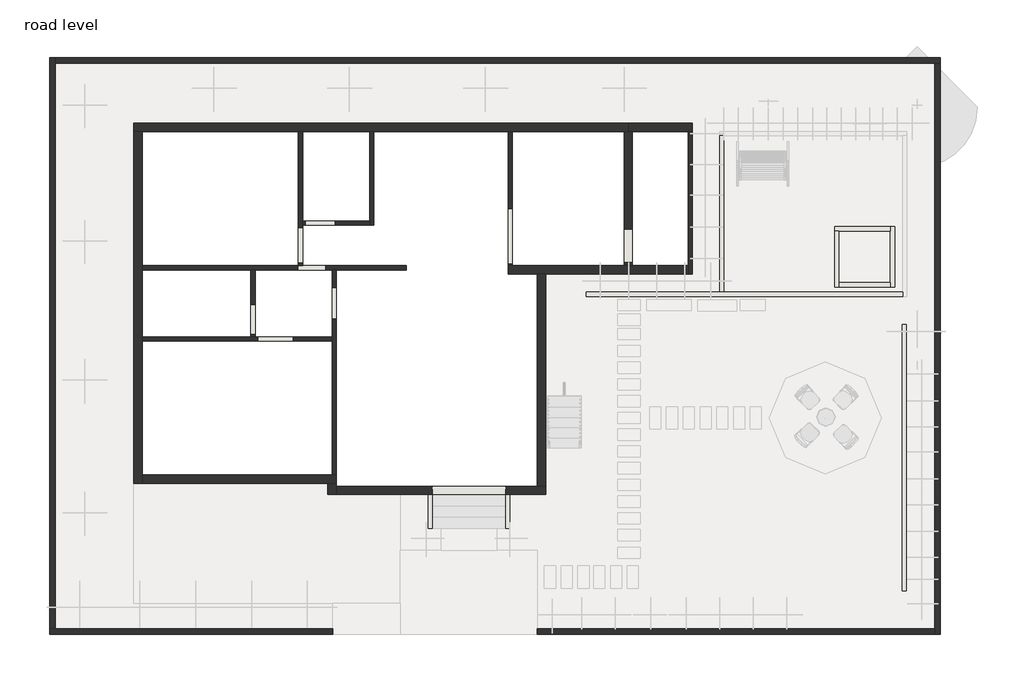
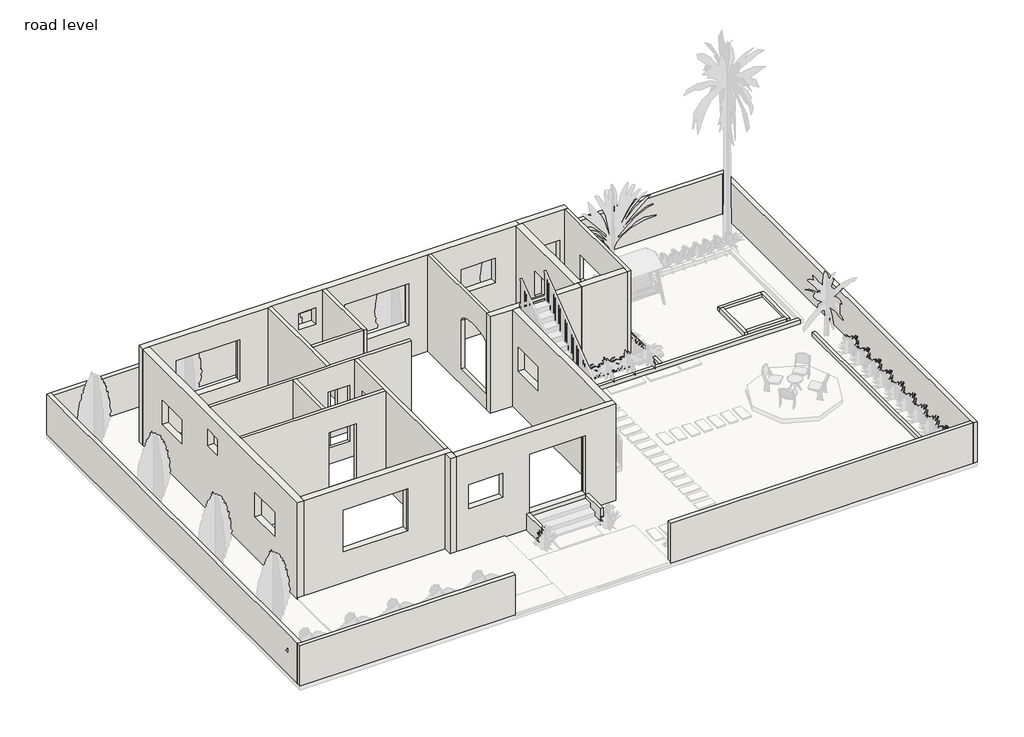
# One storey, part 1 of 3: 33 walls.
"""IFC4 building model written with IfcOpenShell, lengths in millimetres."""

from ifc_helpers import new_model, si_unit, point, frame, origin, origin_with_axes, place, context, project, spatial, polyline, ellipse_curve, trimmed, outline, extrude, faceted_brep, element, save
from ifc_brep_helpers import plane_surface, extruded_surface, advanced_brep

model = new_model("IFC4")

# Units and contexts
model_context = context("Model", 3, world=origin())
ifc_project = project(units=[si_unit("LENGTHUNIT", "METRE", prefix="MILLI")], contexts=[model_context])

# Site, building, storey
site = spatial("IfcSite", under=ifc_project)
building = spatial("IfcBuilding", under=site)
storey = spatial("IfcBuildingStorey", under=building, Name="road level", Elevation=0.0)

# Walls
placement = place(None, origin())
element("IfcWall", 1, ObjectType="Generic - 4.5\"", at=placement, inside=storey, context=model_context, shape_type="Brep", body=[
    faceted_brep([(-13538.1917413, 12365.9965218, 0.0), (-13538.1917413, 8708.3965218, 0.0), (-13538.1917413, 8708.3965218, 3657.6), (-13538.1917413, 12365.9965218, 3657.6), (-13538.1917413, 8778.2465218, 2768.6), (-13538.1917413, 8778.2465218, 609.6), (-13538.1917413, 9743.4465218, 609.6), (-13538.1917413, 9743.4465218, 2768.6), (-13423.8917413, 8708.3965218, 0.0), (-13423.8917413, 9813.2965218, 0.0), (-13423.8917413, 9927.5965218, 0.0), (-13423.8917413, 12365.9965218, 0.0), (-13423.8917413, 12365.9965218, 3657.6), (-13423.8917413, 9927.5965218, 3657.6), (-13423.8917413, 9813.2965218, 3657.6), (-13423.8917413, 8708.3965218, 3657.6), (-13423.8917413, 8778.2465218, 609.6), (-13423.8917413, 8778.2465218, 2768.6), (-13423.8917413, 9743.4465218, 2768.6), (-13423.8917413, 9743.4465218, 609.6)], [[[0, 1, 2, 3], [4, 5, 6, 7]], [[8, 9, 10, 11, 12, 13, 14, 15], [16, 17, 18, 19]], [[1, 0, 11, 10, 9, 8]], [[0, 3, 12, 11]], [[2, 1, 8, 15]], [[16, 5, 4, 17]], [[17, 4, 7, 18]], [[18, 7, 6, 19]], [[5, 16, 19, 6]], [[3, 2, 15, 14, 13, 12]]]),
])
element("IfcWall", 2, ObjectType="Generic - 4.5\"", at=placement, inside=storey, context=model_context, shape_type="Brep", body=[
    faceted_brep([(-10596.8717413, 8708.3965218, 0.0), (-13423.8917413, 8708.3965218, 0.0), (-13538.1917413, 8708.3965218, 0.0), (-17805.3917413, 8708.3965218, 0.0), (-17805.3917413, 8708.3965218, 3657.6), (-13538.1917413, 8708.3965218, 3657.6), (-13423.8917413, 8708.3965218, 3657.6), (-10596.8717413, 8708.3965218, 3657.6), (-12795.2417413, 8708.3965218, 2743.2), (-13557.2417413, 8708.3965218, 2743.2), (-13557.2417413, 8708.3965218, 609.6), (-12795.2417413, 8708.3965218, 609.6), (-10596.8717413, 8594.0965218, 0.0), (-10596.8717413, 8594.0965218, 3657.6), (-12509.4917413, 8594.0965218, 3657.6), (-12623.7917413, 8594.0965218, 3657.6), (-14719.2917413, 8594.0965218, 3657.6), (-14833.5917413, 8594.0965218, 3657.6), (-17805.3917413, 8594.0965218, 3657.6), (-17805.3917413, 8594.0965218, 0.0), (-14833.5917413, 8594.0965218, 0.0), (-14719.2917413, 8594.0965218, 0.0), (-12623.7917413, 8594.0965218, 0.0), (-12509.4917413, 8594.0965218, 0.0), (-12795.2417413, 8594.0965218, 2743.2), (-12795.2417413, 8594.0965218, 609.6), (-13557.2417413, 8594.0965218, 609.6), (-13557.2417413, 8594.0965218, 2743.2)], [[[0, 1, 2, 3, 4, 5, 6, 7], [8, 9, 10, 11]], [[12, 13, 14, 15, 16, 17, 18, 19, 20, 21, 22, 23], [24, 25, 26, 27]], [[3, 2, 1, 0, 12, 23, 22, 21, 20, 19]], [[0, 7, 13, 12]], [[4, 3, 19, 18]], [[25, 24, 8, 11]], [[26, 25, 11, 10]], [[27, 26, 10, 9]], [[24, 27, 9, 8]], [[7, 6, 5, 4, 18, 17, 16, 15, 14, 13]]]),
])
element("IfcWall", 3, ObjectType="Generic - 4.5\"", at=placement, inside=storey, context=model_context, shape_type="Brep", body=[
    faceted_brep([(-11595.0917413, 12365.9965218, 0.0), (-11595.0917413, 9927.5965218, 0.0), (-11595.0917413, 9813.2965218, 0.0), (-11595.0917413, 9813.2965218, 3657.6), (-11595.0917413, 9927.5965218, 3657.6), (-11595.0917413, 12365.9965218, 3657.6), (-11480.7917413, 12365.9965218, 0.0), (-11480.7917413, 12365.9965218, 3657.6), (-11480.7917413, 9813.2965218, 3657.6), (-11480.7917413, 9813.2965218, 0.0)], [[[0, 1, 2, 3, 4, 5]], [[6, 7, 8, 9]], [[2, 1, 0, 6, 9]], [[0, 5, 7, 6]], [[3, 2, 9, 8]], [[5, 4, 3, 8, 7]]]),
])
element("IfcWall", 4, ObjectType="Generic - 4.5\"", at=placement, inside=storey, context=model_context, shape_type="SweptSolid", body=[
    extrude(outline(polyline([(0.0, -11595.0917413), (3657.6, -11595.0917413), (3657.6, -13423.8917413), (0.0, -13423.8917413), (0.0, -11595.0917413)]), holes=[polyline([(609.6, -12541.2417413), (609.6, -13354.0417413), (2743.2, -13354.0417413), (2743.2, -12541.2417413), (609.6, -12541.2417413)])]), frame((0.0, 9813.2965218, 0.0), z_axis=(0.0, 1.0, 0.0), x_axis=(0.0, 0.0, 1.0)), (0.0, 0.0, 1.0), 114.3),
])
element("IfcWall", 5, ObjectType="Generic - 4.5\"", at=placement, inside=storey, context=model_context, shape_type="AdvancedBrep", body=[
    advanced_brep(
    [(-7823.1917413, 12365.9965218, 0.0), (-7823.1917413, 8708.3965218, 0.0), (-7823.1917413, 8708.3965218, 3657.6), (-7823.1917413, 12365.9965218, 3657.6), (-7823.1917413, 8746.4965218, 2438.4), (-7823.1917413, 8746.4965218, 609.6), (-7823.1917413, 10270.4965218, 609.6), (-7823.1917413, 10270.4965218, 2438.4), (-7708.8917413, 12365.9965218, 0.0), (-7708.8917413, 12365.9965218, 3657.6), (-7708.8917413, 8708.3965218, 3657.6), (-7708.8917413, 8708.3965218, 0.0), (-7708.8917413, 8746.4965218, 2438.4), (-7708.8917413, 10270.4965218, 2438.4), (-7708.8917413, 10270.4965218, 609.6), (-7708.8917413, 8746.4965218, 609.6)],
    [
        (0, 1),
        (1, 2),
        (2, 3),
        (3, 0),
        (4, 5),
        (5, 6),
        (6, 7),
        (7, 4, ellipse_curve(frame((-7823.1917413, 9508.4965218, 2438.4), z_axis=(1.0, 0.0, 0.0), x_axis=(0.0, -1.0, 0.0)), 762.0, 304.8)),
        (8, 9),
        (9, 10),
        (10, 11),
        (11, 8),
        (12, 13, ellipse_curve(frame((-7708.8917413, 9508.4965218, 2438.4), z_axis=(-1.0, 0.0, 0.0), x_axis=(0.0, -1.0, 0.0)), 762.0, 304.8)),
        (13, 14),
        (14, 15),
        (15, 12),
        (0, 8),
        (11, 1),
        (3, 9),
        (10, 2),
        (12, 4),
        (7, 13),
        (6, 14),
        (5, 15),
    ],
    [
        plane_surface(frame((-7823.1917413, 12708.8965218, 0.0), z_axis=(-1.0, 0.0, 0.0), x_axis=(0.0, -1.0, 0.0))),
        plane_surface(frame((-7708.8917413, 12708.8965218, 0.0), z_axis=(1.0, 0.0, 0.0), x_axis=(0.0, 1.0, 0.0))),
        plane_surface(frame((-7823.1917413, 12480.2965218, 0.0), z_axis=(0.0, 0.0, -1.0), x_axis=(1.0, 0.0, 0.0))),
        plane_surface(frame((-17805.3917413, 12365.9965218, 0.0), z_axis=(0.0, 1.0, 0.0), x_axis=(1.0, 0.0, 0.0))),
        plane_surface(frame((-4946.6417413, 8708.3965218, 0.0), z_axis=(0.0, -1.0, 0.0), x_axis=(-1.0, 0.0, 0.0))),
        extruded_surface(trimmed(ellipse_curve(frame((-7937.4917413, 9508.4965218, 2438.4), z_axis=(-1.0, 0.0, 0.0), x_axis=(0.0, -1.0, 0.0)), 762.0, 304.8), [point((-7937.4917413, 8746.4965218, 2438.4))], [point((-7937.4917413, 10270.4965218, 2438.4))], True, "CARTESIAN"), (114.30000000000018, 0.0, 0.0), 114.30000000000018),
        plane_surface(frame((-7708.8917413, 10270.4965218, 2438.4), z_axis=(0.0, -1.0, 0.0), x_axis=(-1.0, 0.0, 0.0))),
        plane_surface(frame((-7708.8917413, 10270.4965218, 609.6), z_axis=(0.0, 0.0, 1.0), x_axis=(-1.0, 0.0, 0.0))),
        plane_surface(frame((-7708.8917413, 8746.4965218, 609.6), z_axis=(0.0, 1.0, 0.0), x_axis=(-1.0, 0.0, 0.0))),
        plane_surface(frame((-2241.5417413, 12594.5965218, 3657.6), z_axis=(0.0, 0.0, 1.0), x_axis=(0.0, -1.0, 0.0))),
    ],
    [
        (0, [[1, 2, 3, 4], [5, 6, 7, 8]]),
        (1, [[9, 10, 11, 12], [13, 14, 15, 16]]),
        (2, [[-1, 17, -12, 18]]),
        (3, [[-4, 19, -9, -17]]),
        (4, [[-2, -18, -11, 20]]),
        (5, [[-13, 21, -8, 22]]),
        (6, [[-14, -22, -7, 23]]),
        (7, [[-15, -23, -6, 24]]),
        (8, [[-16, -24, -5, -21]]),
        (9, [[-3, -20, -10, -19]]),
    ],
),
])
element("IfcWall", 6, ObjectType="Generic - 4.5\"", at=placement, inside=storey, context=model_context, shape_type="Brep", body=[
    faceted_brep([(-17805.3917413, 6650.9965218, 0.0), (-12623.7917413, 6650.9965218, 0.0), (-12623.7917413, 6650.9965218, 3657.6), (-17805.3917413, 6650.9965218, 3657.6), (-13684.2417413, 6650.9965218, 2768.6), (-13684.2417413, 6650.9965218, 609.6), (-14649.4417413, 6650.9965218, 609.6), (-14649.4417413, 6650.9965218, 2768.6), (-12623.7917413, 6765.2965218, 0.0), (-14719.2917413, 6765.2965218, 0.0), (-14833.5917413, 6765.2965218, 0.0), (-17805.3917413, 6765.2965218, 0.0), (-17805.3917413, 6765.2965218, 3657.6), (-14833.5917413, 6765.2965218, 3657.6), (-14719.2917413, 6765.2965218, 3657.6), (-12623.7917413, 6765.2965218, 3657.6), (-13684.2417413, 6765.2965218, 609.6), (-13684.2417413, 6765.2965218, 2768.6), (-14649.4417413, 6765.2965218, 2768.6), (-14649.4417413, 6765.2965218, 609.6)], [[[0, 1, 2, 3], [4, 5, 6, 7]], [[8, 9, 10, 11, 12, 13, 14, 15], [16, 17, 18, 19]], [[1, 0, 11, 10, 9, 8]], [[0, 3, 12, 11]], [[2, 1, 8, 15]], [[16, 5, 4, 17]], [[17, 4, 7, 18]], [[18, 7, 6, 19]], [[5, 16, 19, 6]], [[3, 2, 15, 14, 13, 12]]]),
])
element("IfcWall", 7, ObjectType="Generic - 4.5\"", at=placement, inside=storey, context=model_context, shape_type="SweptSolid", body=[
    extrude(outline(polyline([(6765.2965218, 0.0), (6765.2965218, 3657.6), (8594.0965218, 3657.6), (8594.0965218, 0.0), (6765.2965218, 0.0)]), holes=[polyline([(7647.9465218, 609.6), (7647.9465218, 2743.2), (6835.1465218, 2743.2), (6835.1465218, 609.6), (7647.9465218, 609.6)])]), frame((-14833.5917413, 0.0, 0.0), z_axis=(1.0, 0.0, 0.0), x_axis=(0.0, 1.0, 0.0)), (0.0, 0.0, 1.0), 114.3),
])
element("IfcWall", 8, ObjectType="Generic - 4.5\"", at=placement, inside=storey, context=model_context, shape_type="Brep", body=[
    faceted_brep([(-12509.4917413, 2993.3965218, 0.0), (-12509.4917413, 8594.0965218, 0.0), (-12509.4917413, 8594.0965218, 3657.6), (-12509.4917413, 2993.3965218, 3657.6), (-12509.4917413, 7247.8965218, 2743.2), (-12509.4917413, 8111.4965218, 2743.2), (-12509.4917413, 8111.4965218, 609.6), (-12509.4917413, 7247.8965218, 609.6), (-12623.7917413, 2993.3965218, 0.0), (-12623.7917413, 2993.3965218, 3657.6), (-12623.7917413, 6650.9965218, 3657.6), (-12623.7917413, 6765.2965218, 3657.6), (-12623.7917413, 8594.0965218, 3657.6), (-12623.7917413, 8594.0965218, 0.0), (-12623.7917413, 6765.2965218, 0.0), (-12623.7917413, 6650.9965218, 0.0), (-12623.7917413, 7247.8965218, 2743.2), (-12623.7917413, 7247.8965218, 609.6), (-12623.7917413, 8111.4965218, 609.6), (-12623.7917413, 8111.4965218, 2743.2)], [[[0, 1, 2, 3], [4, 5, 6, 7]], [[8, 9, 10, 11, 12, 13, 14, 15], [16, 17, 18, 19]], [[1, 0, 8, 15, 14, 13]], [[0, 3, 9, 8]], [[2, 1, 13, 12]], [[17, 16, 4, 7]], [[18, 17, 7, 6]], [[19, 18, 6, 5]], [[16, 19, 5, 4]], [[3, 2, 12, 11, 10, 9]]]),
])
element("IfcWall", 9, ObjectType="Generic - 4.5\"", at=placement, inside=storey, context=model_context, shape_type="Brep", body=[
    faceted_brep([(-2908.2917413, 12365.9965218, 0.0), (-2908.2917413, 8708.3965218, 0.0), (-2908.2917413, 8479.7965218, 0.0), (-2908.2917413, 8479.7965218, 3657.6), (-2908.2917413, 8708.3965218, 3657.6), (-2908.2917413, 12365.9965218, 3657.6), (-2908.2917413, 10194.2965218, 2489.2), (-2908.2917413, 10194.2965218, 1574.8), (-2908.2917413, 11413.4965218, 1574.8), (-2908.2917413, 11413.4965218, 2489.2), (-2793.9917413, 12365.9965218, 0.0), (-2793.9917413, 12365.9965218, 3657.6), (-2793.9917413, 8479.7965218, 3657.6), (-2793.9917413, 8479.7965218, 0.0), (-2793.9917413, 10194.2965218, 2489.2), (-2793.9917413, 11413.4965218, 2489.2), (-2793.9917413, 11413.4965218, 1574.8), (-2793.9917413, 10194.2965218, 1574.8)], [[[0, 1, 2, 3, 4, 5], [6, 7, 8, 9]], [[10, 11, 12, 13], [14, 15, 16, 17]], [[2, 1, 0, 10, 13]], [[3, 2, 13, 12]], [[0, 5, 11, 10]], [[7, 6, 14, 17]], [[8, 7, 17, 16]], [[9, 8, 16, 15]], [[6, 9, 15, 14]], [[5, 4, 3, 12, 11]]]),
])
element("IfcWall", 10, ObjectType="Generic - 4.5\"", at=placement, inside=storey, context=model_context, shape_type="Brep", body=[
    faceted_brep([(2940.0582587, 7984.4965218, 0.0), (-1936.7417413, 7984.4965218, 0.0), (-2051.0417413, 7984.4965218, 0.0), (-5689.5917413, 7984.4965218, 0.0), (-5689.5917413, 7984.4965218, 152.4), (-2051.0417413, 7984.4965218, 152.4), (-1936.7417413, 7984.4965218, 152.4), (2940.0582587, 7984.4965218, 152.4), (2940.0582587, 7870.1965218, 0.0), (2940.0582587, 7870.1965218, 152.4), (-5689.5917413, 7870.1965218, 152.4), (-5689.5917413, 7870.1965218, 0.0)], [[[0, 1, 2, 3, 4, 5, 6, 7]], [[8, 9, 10, 11]], [[3, 2, 1, 0, 8, 11]], [[4, 3, 11, 10]], [[7, 6, 5, 4, 10, 9]], [[0, 7, 9, 8]]]),
])
element("IfcWall", 11, ObjectType="Generic - 4.5\"", at=placement, inside=storey, context=model_context, shape_type="SweptSolid", body=[
    extrude(outline(polyline([(-1936.7417413, 12251.6965218), (-1936.7417413, 7984.4965218), (-2051.0417413, 7984.4965218), (-2051.0417413, 12251.6965218), (-1936.7417413, 12251.6965218)])), origin_with_axes(), (0.0, 0.0, 1.0), 152.4),
])
element("IfcWall", 12, ObjectType="Generic - 4.5\"", at=placement, inside=storey, context=model_context, shape_type="SweptSolid", body=[
    extrude(outline(polyline([(2921.0082587, -158.6328583), (2921.0082587, 7101.8465218), (3035.3082587, 7101.8465218), (3035.3082587, -158.6328583), (2921.0082587, -158.6328583)])), origin_with_axes(), (0.0, 0.0, 1.0), 152.4),
])
element("IfcWall", 13, ObjectType="Generic - 4.5\"", at=placement, inside=storey, context=model_context, shape_type="SweptSolid", body=[
    extrude(outline(polyline([(-10004.2917413, 1545.5965218), (-10004.2917413, 2459.9965218), (-9889.9917413, 2459.9965218), (-9889.9917413, 1545.5965218), (-10004.2917413, 1545.5965218)])), origin_with_axes(), (0.0, 0.0, 1.0), 609.6),
])
element("IfcWall", 14, ObjectType="Generic - 4.5\"", at=placement, inside=storey, context=model_context, shape_type="SweptSolid", body=[
    extrude(outline(polyline([(-7888.5983292, 1545.5965218), (-7888.5983292, 2459.9965218), (-7774.2983292, 2459.9965218), (-7774.2983292, 1545.5965218), (-7888.5983292, 1545.5965218)])), origin_with_axes(), (0.0, 0.0, 1.0), 609.6),
])
element("IfcWall", 15, ObjectType="Generic - 4.5\"", at=placement, inside=storey, context=model_context, shape_type="Brep", body=[
    faceted_brep([(2719.3138793, 8130.4970238, 0.0), (2719.3138793, 9768.7970238, 0.0), (2719.3138793, 9768.7970238, 152.4), (2719.3138793, 8130.4970238, 152.4), (2605.0138793, 8130.4970238, 0.0), (2605.0138793, 8130.4970238, 152.4), (2605.0138793, 8244.7970238, 152.4), (2605.0138793, 9654.4970238, 152.4), (2605.0138793, 9768.7970238, 152.4), (2605.0138793, 9768.7970238, 0.0), (2605.0138793, 9654.4970238, 0.0), (2605.0138793, 8244.7970238, 0.0)], [[[0, 1, 2, 3]], [[4, 5, 6, 7, 8, 9, 10, 11]], [[1, 0, 4, 11, 10, 9]], [[3, 2, 8, 7, 6, 5]], [[2, 1, 9, 8]], [[0, 3, 5, 4]]]),
])
element("IfcWall", 16, ObjectType="Generic - 4.5\"", at=placement, inside=storey, context=model_context, shape_type="Brep", body=[
    faceted_brep([(2605.0138793, 9768.7970238, 0.0), (1081.0138793, 9768.7970238, 0.0), (1081.0138793, 9768.7970238, 152.4), (2605.0138793, 9768.7970238, 152.4), (2605.0138793, 9654.4970238, 0.0), (2605.0138793, 9654.4970238, 152.4), (1195.3138793, 9654.4970238, 152.4), (1081.0138793, 9654.4970238, 152.4), (1081.0138793, 9654.4970238, 0.0), (1195.3138793, 9654.4970238, 0.0)], [[[0, 1, 2, 3]], [[4, 5, 6, 7, 8, 9]], [[1, 0, 4, 9, 8]], [[3, 2, 7, 6, 5]], [[0, 3, 5, 4]], [[2, 1, 8, 7]]]),
])
element("IfcWall", 17, ObjectType="Generic - 4.5\"", at=placement, inside=storey, context=model_context, shape_type="Brep", body=[
    faceted_brep([(1081.0138793, 9654.4970238, 0.0), (1081.0138793, 8130.4970238, 0.0), (1081.0138793, 8130.4970238, 152.4), (1081.0138793, 9654.4970238, 152.4), (1195.3138793, 9654.4970238, 0.0), (1195.3138793, 9654.4970238, 152.4), (1195.3138793, 8244.7970238, 152.4), (1195.3138793, 8130.4970238, 152.4), (1195.3138793, 8130.4970238, 0.0), (1195.3138793, 8244.7970238, 0.0)], [[[0, 1, 2, 3]], [[4, 5, 6, 7, 8, 9]], [[1, 0, 4, 9, 8]], [[3, 2, 7, 6, 5]], [[0, 3, 5, 4]], [[2, 1, 8, 7]]]),
])
element("IfcWall", 18, ObjectType="Generic - 4.5\"", at=placement, inside=storey, context=model_context, shape_type="SweptSolid", body=[
    extrude(outline(polyline([(2605.0138793, 8130.4970238), (1195.3138793, 8130.4970238), (1195.3138793, 8244.7970238), (2605.0138793, 8244.7970238), (2605.0138793, 8130.4970238)])), origin_with_axes(), (0.0, 0.0, 1.0), 152.4),
])
element("IfcWall", 19, ObjectType="Generic - 6\"", at=placement, inside=storey, context=model_context, shape_type="Brep", body=[
    faceted_brep([(-20167.5917413, 14232.8965218, 0.0), (3816.3582587, 14232.8965218, 0.0), (3968.7582587, 14232.8965218, 0.0), (3968.7582587, 14232.8965218, 1524.0), (3816.3582587, 14232.8965218, 1524.0), (-20167.5917413, 14232.8965218, 1524.0), (-20167.5917413, 14385.2965218, 0.0), (-20167.5917413, 14385.2965218, 1524.0), (3968.7582587, 14385.2965218, 1524.0), (3968.7582587, 14385.2965218, 0.0)], [[[0, 1, 2, 3, 4, 5]], [[6, 7, 8, 9]], [[2, 1, 0, 6, 9]], [[5, 4, 3, 8, 7]], [[3, 2, 9, 8]], [[0, 5, 7, 6]]]),
])
element("IfcWall", 20, ObjectType="Generic - 6\"", at=placement, inside=storey, context=model_context, shape_type="Brep", body=[
    faceted_brep([(3816.3582587, 14232.8965218, 0.0), (3816.3582587, -1197.6034782, 0.0), (3816.3582587, -1350.0034782, 0.0), (3816.3582587, -1350.0034782, 1524.0), (3816.3582587, -1197.6034782, 1524.0), (3816.3582587, 14232.8965218, 1524.0), (3968.7582587, 14232.8965218, 0.0), (3968.7582587, 14232.8965218, 1524.0), (3968.7582587, -1350.0034782, 1524.0), (3968.7582587, -1350.0034782, 0.0)], [[[0, 1, 2, 3, 4, 5]], [[6, 7, 8, 9]], [[2, 1, 0, 6, 9]], [[5, 4, 3, 8, 7]], [[0, 5, 7, 6]], [[3, 2, 9, 8]]]),
])
element("IfcWall", 21, ObjectType="Generic - 6\"", at=placement, inside=storey, context=model_context, shape_type="SweptSolid", body=[
    extrude(outline(polyline([(-7023.0917413, -1197.6034782), (3816.3582587, -1197.6034782), (3816.3582587, -1350.0034782), (-7023.0917413, -1350.0034782), (-7023.0917413, -1197.6034782)])), origin_with_axes(), (0.0, 0.0, 1.0), 1524.0),
])
element("IfcWall", 22, ObjectType="Generic - 6\"", at=placement, inside=storey, context=model_context, shape_type="Brep", body=[
    faceted_brep([(-20167.5917413, -1197.6034782, 0.0), (-20167.5917413, 14232.8965218, 0.0), (-20167.5917413, 14385.2965218, 0.0), (-20167.5917413, 14385.2965218, 1524.0), (-20167.5917413, 14232.8965218, 1524.0), (-20167.5917413, -1197.6034782, 1524.0), (-20319.9917413, -1197.6034782, 0.0), (-20319.9917413, -1197.6034782, 1524.0), (-20319.9917413, 14385.2965218, 1524.0), (-20319.9917413, 14385.2965218, 0.0)], [[[0, 1, 2, 3, 4, 5]], [[6, 7, 8, 9]], [[2, 1, 0, 6, 9]], [[5, 4, 3, 8, 7]], [[0, 5, 7, 6]], [[3, 2, 9, 8]]]),
])
element("IfcWall", 23, ObjectType="Generic - 6\"", at=placement, inside=storey, context=model_context, shape_type="Brep", body=[
    faceted_brep([(-12598.3917413, -1197.6034782, 0.0), (-20167.5917413, -1197.6034782, 0.0), (-20319.9917413, -1197.6034782, 0.0), (-20319.9917413, -1197.6034782, 1524.0), (-20167.5917413, -1197.6034782, 1524.0), (-12598.3917413, -1197.6034782, 1524.0), (-12598.3917413, -1350.0034782, 0.0), (-12598.3917413, -1350.0034782, 1524.0), (-20319.9917413, -1350.0034782, 1524.0), (-20319.9917413, -1350.0034782, 0.0)], [[[0, 1, 2, 3, 4, 5]], [[6, 7, 8, 9]], [[2, 1, 0, 6, 9]], [[5, 4, 3, 8, 7]], [[0, 5, 7, 6]], [[3, 2, 9, 8]]]),
])
element("IfcWall", 24, ObjectType="Generic - 9\"", at=placement, inside=storey, context=model_context, shape_type="Brep", body=[
    faceted_brep([(-18033.9917413, 12365.9965218, 0.0), (-17805.3917413, 12365.9965218, 0.0), (-13538.1917413, 12365.9965218, 0.0), (-13423.8917413, 12365.9965218, 0.0), (-11595.0917413, 12365.9965218, 0.0), (-11480.7917413, 12365.9965218, 0.0), (-7823.1917413, 12365.9965218, 0.0), (-7708.8917413, 12365.9965218, 0.0), (-4660.8917413, 12365.9965218, 0.0), (-4546.5917413, 12365.9965218, 0.0), (-4546.5917413, 12365.9965218, 3657.6), (-4660.8917413, 12365.9965218, 3657.6), (-7708.8917413, 12365.9965218, 3657.6), (-7823.1917413, 12365.9965218, 3657.6), (-11480.7917413, 12365.9965218, 3657.6), (-11595.0917413, 12365.9965218, 3657.6), (-13423.8917413, 12365.9965218, 3657.6), (-13538.1917413, 12365.9965218, 3657.6), (-17805.3917413, 12365.9965218, 3657.6), (-18033.9917413, 12365.9965218, 3657.6), (-16843.3667413, 12365.9965218, 2794.0), (-14557.3667413, 12365.9965218, 2794.0), (-14557.3667413, 12365.9965218, 1219.2), (-16843.3667413, 12365.9965218, 1219.2), (-10794.9917413, 12365.9965218, 2794.0), (-8508.9917413, 12365.9965218, 2794.0), (-8508.9917413, 12365.9965218, 1219.2), (-10794.9917413, 12365.9965218, 1219.2), (-5394.3167413, 12365.9965218, 2667.0), (-5394.3167413, 12365.9965218, 1752.6), (-6613.5167413, 12365.9965218, 1752.6), (-6613.5167413, 12365.9965218, 2667.0), (-12452.3417413, 12365.9965218, 3048.0), (-11842.7417413, 12365.9965218, 3048.0), (-11842.7417413, 12365.9965218, 2438.4), (-12452.3417413, 12365.9965218, 2438.4), (-18033.9917413, 12594.5965218, 0.0), (-18033.9917413, 12594.5965218, 3657.6), (-4546.5917413, 12594.5965218, 3657.6), (-4546.5917413, 12594.5965218, 0.0), (-14545.2374161, 12594.5965218, 2794.0), (-16855.4960665, 12594.5965218, 2794.0), (-16855.4960665, 12594.5965218, 1219.2), (-14545.2374161, 12594.5965218, 1219.2), (-8496.8624161, 12594.5965218, 2794.0), (-10807.1210665, 12594.5965218, 2794.0), (-10807.1210665, 12594.5965218, 1219.2), (-8496.8624161, 12594.5965218, 1219.2), (-5394.3167413, 12594.5965218, 2667.0), (-6613.5167413, 12594.5965218, 2667.0), (-6613.5167413, 12594.5965218, 1752.6), (-5394.3167413, 12594.5965218, 1752.6), (-12452.3417413, 12594.5965218, 3048.0), (-12452.3417413, 12594.5965218, 2438.4), (-11842.7417413, 12594.5965218, 2438.4), (-11842.7417413, 12594.5965218, 3048.0), (-16843.3667413, 12525.8077002, 2794.0), (-14557.3667413, 12525.8077003, 2794.0), (-16843.3667413, 12525.8077002, 1219.2), (-14557.3667413, 12525.8077003, 1219.2), (-10794.9917413, 12525.8077002, 2794.0), (-8508.9917413, 12525.8077002, 2794.0), (-10794.9917413, 12525.8077002, 1219.2), (-8508.9917413, 12525.8077002, 1219.2)], [[[0, 1, 2, 3, 4, 5, 6, 7, 8, 9, 10, 11, 12, 13, 14, 15, 16, 17, 18, 19], [20, 21, 22, 23], [24, 25, 26, 27], [28, 29, 30, 31], [32, 33, 34, 35]], [[36, 37, 38, 39], [40, 41, 42, 43], [44, 45, 46, 47], [48, 49, 50, 51], [52, 53, 54, 55]], [[9, 8, 7, 6, 5, 4, 3, 2, 1, 0, 36, 39]], [[10, 9, 39, 38]], [[0, 19, 37, 36]], [[56, 41, 40, 57, 21, 20]], [[58, 23, 22, 59, 43, 42]], [[56, 20, 23, 58]], [[21, 57, 59, 22]], [[57, 40, 43, 59]], [[41, 56, 58, 42]], [[60, 45, 44, 61, 25, 24]], [[62, 27, 26, 63, 47, 46]], [[60, 24, 27, 62]], [[25, 61, 63, 26]], [[61, 44, 47, 63]], [[45, 60, 62, 46]], [[29, 28, 48, 51]], [[30, 29, 51, 50]], [[31, 30, 50, 49]], [[28, 31, 49, 48]], [[53, 52, 32, 35]], [[54, 53, 35, 34]], [[55, 54, 34, 33]], [[52, 55, 33, 32]], [[19, 18, 17, 16, 15, 14, 13, 12, 11, 10, 38, 37]]]),
])
element("IfcWall", 25, ObjectType="Generic - 9\"", at=placement, inside=storey, context=model_context, shape_type="Brep", body=[
    faceted_brep([(-18033.9917413, 12365.9965218, 0.0), (-18033.9917413, 2764.7965218, 0.0), (-18033.9917413, 2764.7965218, 3657.6), (-18033.9917413, 12365.9965218, 3657.6), (-18033.9917413, 5403.2215218, 2438.4), (-18033.9917413, 4184.0215218, 2438.4), (-18033.9917413, 4184.0215218, 1524.0), (-18033.9917413, 5403.2215218, 1524.0), (-18033.9917413, 11175.3715218, 2438.4), (-18033.9917413, 9956.1715218, 2438.4), (-18033.9917413, 9956.1715218, 1524.0), (-18033.9917413, 11175.3715218, 1524.0), (-18033.9917413, 7736.8465218, 3048.0), (-18033.9917413, 7736.8465218, 2438.4), (-18033.9917413, 8346.4465218, 2438.4), (-18033.9917413, 8346.4465218, 3048.0), (-17805.3917413, 12365.9965218, 0.0), (-17805.3917413, 12365.9965218, 3657.6), (-17805.3917413, 8708.3965218, 3657.6), (-17805.3917413, 8594.0965218, 3657.6), (-17805.3917413, 6765.2965218, 3657.6), (-17805.3917413, 6650.9965218, 3657.6), (-17805.3917413, 2993.3965218, 3657.6), (-17805.3917413, 2764.7965218, 3657.6), (-17805.3917413, 2764.7965218, 0.0), (-17805.3917413, 2993.3965218, 0.0), (-17805.3917413, 6650.9965218, 0.0), (-17805.3917413, 6765.2965218, 0.0), (-17805.3917413, 8594.0965218, 0.0), (-17805.3917413, 8708.3965218, 0.0), (-17805.3917413, 5403.2215218, 2438.4), (-17805.3917413, 5403.2215218, 1524.0), (-17805.3917413, 4184.0215218, 1524.0), (-17805.3917413, 4184.0215218, 2438.4), (-17805.3917413, 11175.3715218, 2438.4), (-17805.3917413, 11175.3715218, 1524.0), (-17805.3917413, 9956.1715218, 1524.0), (-17805.3917413, 9956.1715218, 2438.4), (-17805.3917413, 7736.8465218, 3048.0), (-17805.3917413, 8346.4465218, 3048.0), (-17805.3917413, 8346.4465218, 2438.4), (-17805.3917413, 7736.8465218, 2438.4)], [[[0, 1, 2, 3], [4, 5, 6, 7], [8, 9, 10, 11], [12, 13, 14, 15]], [[16, 17, 18, 19, 20, 21, 22, 23, 24, 25, 26, 27, 28, 29], [30, 31, 32, 33], [34, 35, 36, 37], [38, 39, 40, 41]], [[1, 0, 16, 29, 28, 27, 26, 25, 24]], [[0, 3, 17, 16]], [[2, 1, 24, 23]], [[31, 30, 4, 7]], [[32, 31, 7, 6]], [[33, 32, 6, 5]], [[30, 33, 5, 4]], [[35, 34, 8, 11]], [[36, 35, 11, 10]], [[37, 36, 10, 9]], [[34, 37, 9, 8]], [[13, 12, 38, 41]], [[14, 13, 41, 40]], [[15, 14, 40, 39]], [[12, 15, 39, 38]], [[3, 2, 23, 22, 21, 20, 19, 18, 17]]]),
])
element("IfcWall", 26, ObjectType="Generic - 9\"", at=placement, inside=storey, context=model_context, shape_type="Brep", body=[
    faceted_brep([(-4660.8917413, 12365.9965218, 0.0), (-4660.8917413, 8708.3965218, 0.0), (-4660.8917413, 8708.3965218, 3657.6), (-4660.8917413, 12365.9965218, 3657.6), (-4660.8917413, 8797.2965218, 2768.6), (-4660.8917413, 8797.2965218, 609.6), (-4660.8917413, 9711.6965218, 609.6), (-4660.8917413, 9711.6965218, 2768.6), (-4660.8917413, 9965.6965218, 2641.6), (-4660.8917413, 9965.6965218, 1727.2), (-4660.8917413, 11184.8965218, 1727.2), (-4660.8917413, 11184.8965218, 2641.6), (-4432.2917413, 8708.3965218, 0.0), (-4432.2917413, 12365.9965218, 0.0), (-4432.2917413, 12365.9965218, 3657.6), (-4432.2917413, 8708.3965218, 3657.6), (-4432.2917413, 8797.2965218, 609.6), (-4432.2917413, 8797.2965218, 2768.6), (-4432.2917413, 9711.6965218, 2768.6), (-4432.2917413, 9711.6965218, 609.6), (-4432.2917413, 9965.6965218, 1727.2), (-4432.2917413, 9965.6965218, 2641.6), (-4432.2917413, 11184.8965218, 2641.6), (-4432.2917413, 11184.8965218, 1727.2), (-4546.5917413, 12365.9965218, 0.0), (-4546.5917413, 8708.3965218, 0.0), (-4546.5917413, 12365.9965218, 3657.6), (-4546.5917413, 8708.3965218, 3657.6)], [[[0, 1, 2, 3], [4, 5, 6, 7], [8, 9, 10, 11]], [[12, 13, 14, 15], [16, 17, 18, 19], [20, 21, 22, 23]], [[1, 0, 24, 13, 12, 25]], [[16, 5, 4, 17]], [[17, 4, 7, 18]], [[18, 7, 6, 19]], [[5, 16, 19, 6]], [[9, 8, 21, 20]], [[10, 9, 20, 23]], [[11, 10, 23, 22]], [[8, 11, 22, 21]], [[0, 3, 26, 14, 13, 24]], [[2, 1, 25, 12, 15, 27]], [[3, 2, 27, 15, 14, 26]]]),
])
element("IfcWall", 27, ObjectType="Generic - 9\"", at=placement, inside=storey, context=model_context, shape_type="Brep", body=[
    faceted_brep([(-2908.2917413, 8708.3965218, 0.0), (-4432.2917413, 8708.3965218, 0.0), (-4546.5917413, 8708.3965218, 0.0), (-4546.5917413, 8708.3965218, 3657.6), (-4432.2917413, 8708.3965218, 3657.6), (-2908.2917413, 8708.3965218, 3657.6), (-2908.2917413, 8479.7965218, 0.0), (-2908.2917413, 8479.7965218, 3657.6), (-4546.5917413, 8479.7965218, 3657.6), (-4546.5917413, 8479.7965218, 0.0)], [[[0, 1, 2, 3, 4, 5]], [[6, 7, 8, 9]], [[2, 1, 0, 6, 9]], [[3, 2, 9, 8]], [[0, 5, 7, 6]], [[5, 4, 3, 8, 7]]]),
])
element("IfcWall", 28, ObjectType="Generic - 9\"", at=placement, inside=storey, context=model_context, shape_type="Brep", body=[
    faceted_brep([(-17805.3917413, 2764.7965218, 0.0), (-12738.0917413, 2764.7965218, 0.0), (-12509.4917413, 2764.7965218, 0.0), (-12509.4917413, 2764.7965218, 3657.6), (-12738.0917413, 2764.7965218, 3657.6), (-17805.3917413, 2764.7965218, 3657.6), (-16398.2960665, 2764.7965218, 2794.0), (-14088.0374161, 2764.7965218, 2794.0), (-14088.0374161, 2764.7965218, 1219.2), (-16398.2960665, 2764.7965218, 1219.2), (-17805.3917413, 2993.3965218, 0.0), (-17805.3917413, 2993.3965218, 3657.6), (-12623.7917413, 2993.3965218, 3657.6), (-12509.4917413, 2993.3965218, 3657.6), (-12509.4917413, 2993.3965218, 0.0), (-12623.7917413, 2993.3965218, 0.0), (-14100.1667413, 2993.3965218, 2794.0), (-16386.1667413, 2993.3965218, 2794.0), (-16386.1667413, 2993.3965218, 1219.2), (-14100.1667413, 2993.3965218, 1219.2), (-14100.1667413, 2833.5853433, 2794.0), (-16386.1667413, 2833.5853433, 2794.0), (-14100.1667413, 2833.5853433, 1219.2), (-16386.1667413, 2833.5853433, 1219.2)], [[[0, 1, 2, 3, 4, 5], [6, 7, 8, 9]], [[10, 11, 12, 13, 14, 15], [16, 17, 18, 19]], [[2, 1, 0, 10, 15, 14]], [[3, 2, 14, 13]], [[0, 5, 11, 10]], [[20, 7, 6, 21, 17, 16]], [[22, 19, 18, 23, 9, 8]], [[20, 16, 19, 22]], [[17, 21, 23, 18]], [[21, 6, 9, 23]], [[7, 20, 22, 8]], [[5, 4, 3, 13, 12, 11]]]),
])
element("IfcWall", 29, ObjectType="Generic - 9\"", at=placement, inside=storey, context=model_context, shape_type="Brep", body=[
    faceted_brep([(-12738.0917413, 2764.7965218, 0.0), (-12738.0917413, 2459.9965218, 0.0), (-12738.0917413, 2459.9965218, 3657.6), (-12738.0917413, 2764.7965218, 3657.6), (-12509.4917413, 2764.7965218, 0.0), (-12509.4917413, 2764.7965218, 3657.6), (-12509.4917413, 2688.5965218, 3657.6), (-12509.4917413, 2459.9965218, 3657.6), (-12509.4917413, 2459.9965218, 0.0), (-12509.4917413, 2688.5965218, 0.0)], [[[0, 1, 2, 3]], [[4, 5, 6, 7, 8, 9]], [[1, 0, 4, 9, 8]], [[0, 3, 5, 4]], [[2, 1, 8, 7]], [[3, 2, 7, 6, 5]]]),
])
element("IfcWall", 30, ObjectType="Generic - 9\"", at=placement, inside=storey, context=model_context, shape_type="Brep", body=[
    faceted_brep([(-12509.4917413, 2459.9965218, 0.0), (-10004.2917413, 2459.9965218, 0.0), (-9889.9917413, 2459.9965218, 0.0), (-7888.5983292, 2459.9965218, 0.0), (-7774.2983292, 2459.9965218, 0.0), (-6794.4917413, 2459.9965218, 0.0), (-6794.4917413, 2459.9965218, 3657.6), (-12509.4917413, 2459.9965218, 3657.6), (-9889.9917413, 2459.9965218, 2818.6), (-7889.9917413, 2459.9965218, 2818.6), (-7889.9917413, 2459.9965218, 609.6), (-9889.9917413, 2459.9965218, 609.6), (-12064.9917413, 2459.9965218, 1524.0), (-12064.9917413, 2459.9965218, 2438.4), (-10845.7917413, 2459.9965218, 2438.4), (-10845.7917413, 2459.9965218, 1524.0), (-6794.4917413, 2688.5965218, 0.0), (-7023.0917413, 2688.5965218, 0.0), (-12509.4917413, 2688.5965218, 0.0), (-12509.4917413, 2688.5965218, 3657.6), (-7023.0917413, 2688.5965218, 3657.6), (-6794.4917413, 2688.5965218, 3657.6), (-7889.9917413, 2688.5965218, 2818.6), (-9889.9917413, 2688.5965218, 2818.6), (-9889.9917413, 2688.5965218, 609.6), (-7889.9917413, 2688.5965218, 609.6), (-12064.9917413, 2688.5965218, 2438.4), (-12064.9917413, 2688.5965218, 1524.0), (-10845.7917413, 2688.5965218, 1524.0), (-10845.7917413, 2688.5965218, 2438.4), (-7889.9917413, 2668.5965218, 2818.6), (-9889.9917413, 2668.5965218, 2818.6), (-9889.9917413, 2598.5965218, 2818.6), (-7889.9917413, 2598.5965218, 2818.6), (-7889.9917413, 2598.5965218, 609.6), (-7874.9917413, 2598.5965218, 609.6), (-7874.9917413, 2668.5965218, 609.6), (-7889.9917413, 2668.5965218, 609.6), (-9889.9917413, 2668.5965218, 609.6), (-9904.9917413, 2668.5965218, 609.6), (-9904.9917413, 2598.5965218, 609.6), (-9889.9917413, 2598.5965218, 609.6), (-9904.9917413, 2598.5965218, 2833.6), (-7874.9917413, 2598.5965218, 2833.6), (-7874.9917413, 2668.5965218, 2833.6), (-9904.9917413, 2668.5965218, 2833.6)], [[[0, 1, 2, 3, 4, 5, 6, 7], [8, 9, 10, 11], [12, 13, 14, 15]], [[16, 17, 18, 19, 20, 21], [22, 23, 24, 25], [26, 27, 28, 29]], [[5, 4, 3, 2, 1, 0, 18, 17, 16]], [[0, 7, 19, 18]], [[6, 5, 16, 21]], [[30, 31, 23, 22]], [[32, 33, 9, 8]], [[34, 35, 36, 37, 25, 24, 38, 39, 40, 41, 11, 10]], [[41, 32, 8, 11]], [[33, 34, 10, 9]], [[33, 32, 41, 40, 42, 43, 35, 34]], [[36, 35, 43, 44]], [[31, 30, 37, 36, 44, 45, 39, 38]], [[37, 30, 22, 25]], [[31, 38, 24, 23]], [[40, 39, 45, 42]], [[43, 42, 45, 44]], [[27, 26, 13, 12]], [[28, 27, 12, 15]], [[29, 28, 15, 14]], [[26, 29, 14, 13]], [[7, 6, 21, 20, 19]]]),
])
element("IfcWall", 31, ObjectType="Generic - 9\"", at=placement, inside=storey, context=model_context, shape_type="SweptSolid", body=[
    extrude(outline(polyline([(2688.5965218, 0.0), (2688.5965218, 3657.6), (8479.7965218, 3657.6), (8479.7965218, 0.0), (2688.5965218, 0.0)]), holes=[polyline([(6917.6965218, 2438.4), (6917.6965218, 1524.0), (8136.8965218, 1524.0), (8136.8965218, 2438.4), (6917.6965218, 2438.4)]), polyline([(3031.4965218, 2438.4), (3031.4965218, 1524.0), (4250.6965218, 1524.0), (4250.6965218, 2438.4), (3031.4965218, 2438.4)])]), frame((-7023.0917413, 0.0, 0.0), z_axis=(1.0, 0.0, 0.0), x_axis=(0.0, 1.0, 0.0)), (0.0, 0.0, 1.0), 228.6),
])
element("IfcWall", 32, ObjectType="Generic - 9\"", at=placement, inside=storey, context=model_context, shape_type="Brep", body=[
    faceted_brep([(-4546.5917413, 12365.9965218, 0.0), (-4432.2917413, 12365.9965218, 0.0), (-2908.2917413, 12365.9965218, 0.0), (-2793.9917413, 12365.9965218, 0.0), (-2793.9917413, 12365.9965218, 3657.6), (-2908.2917413, 12365.9965218, 3657.6), (-4432.2917413, 12365.9965218, 3657.6), (-4546.5917413, 12365.9965218, 3657.6), (-3089.2667413, 12365.9965218, 2540.0), (-3089.2667413, 12365.9965218, 1625.6), (-4308.4667413, 12365.9965218, 1625.6), (-4308.4667413, 12365.9965218, 2540.0), (-4546.5917413, 12594.5965218, 0.0), (-4546.5917413, 12594.5965218, 3657.6), (-2793.9917413, 12594.5965218, 3657.6), (-2793.9917413, 12594.5965218, 0.0), (-3089.2667413, 12594.5965218, 2540.0), (-4308.4667413, 12594.5965218, 2540.0), (-4308.4667413, 12594.5965218, 1625.6), (-3089.2667413, 12594.5965218, 1625.6)], [[[0, 1, 2, 3, 4, 5, 6, 7], [8, 9, 10, 11]], [[12, 13, 14, 15], [16, 17, 18, 19]], [[3, 2, 1, 0, 12, 15]], [[0, 7, 13, 12]], [[4, 3, 15, 14]], [[9, 8, 16, 19]], [[10, 9, 19, 18]], [[11, 10, 18, 17]], [[8, 11, 17, 16]], [[7, 6, 5, 4, 14, 13]]]),
])
element("IfcWall", 33, ObjectType="Generic - 9\"", at=placement, inside=storey, context=model_context, shape_type="Brep", body=[
    faceted_brep([(-4546.5917413, 8708.3965218, 0.0), (-4660.8917413, 8708.3965218, 0.0), (-7708.8917413, 8708.3965218, 0.0), (-7823.1917413, 8708.3965218, 0.0), (-7823.1917413, 8708.3965218, 3657.6), (-7708.8917413, 8708.3965218, 3657.6), (-4660.8917413, 8708.3965218, 3657.6), (-4546.5917413, 8708.3965218, 3657.6), (-4546.5917413, 8479.7965218, 0.0), (-4546.5917413, 8479.7965218, 3657.6), (-6794.4917413, 8479.7965218, 3657.6), (-7023.0917413, 8479.7965218, 3657.6), (-7823.1917413, 8479.7965218, 3657.6), (-7823.1917413, 8479.7965218, 0.0), (-7023.0917413, 8479.7965218, 0.0), (-6794.4917413, 8479.7965218, 0.0)], [[[0, 1, 2, 3, 4, 5, 6, 7]], [[8, 9, 10, 11, 12, 13, 14, 15]], [[3, 2, 1, 0, 8, 15, 14, 13]], [[0, 7, 9, 8]], [[4, 3, 13, 12]], [[7, 6, 5, 4, 12, 11, 10, 9]]]),
])

save(model, "model.ifc")

# Revit data of these elements
# Type "Generic - 4.5\""
#   Assembly Code = "B2010"
#   Layers, outside or top first: 0' - 4 1/2" no material (function 1)
# Type "Generic - 6\""
#   Assembly Code = "B2010"
#   Layers, outside or top first: 0' - 6" no material (function 1)
# Type "Generic - 9\""
#   Assembly Code = "B2010"
#   Layers, outside or top first: 0' - 9" no material (function 1)
# Elements 1, 2, 3, 4, 5, 6, 7, 8 (IfcWall, "Generic - 4.5\"")
#   Top Offset = 0' - 0"
#   Base Offset = 0' - 0"
#   wall height = 12' - 0"
#   Phase Created = New Construction
#   Base Constraint = road level
#   Top Constraint = terrace
#   Materials on its faces: "Default Wall"
# Element 9 (IfcWall, "Generic - 4.5\"")
#   Top Offset = 0' - 0"
#   Base Offset = 0' - 0"
#   wall height = 12' - 0"
#   Phase Created = New Construction
#   Base Constraint = road level
#   Top Constraint = terrace
#   Materials on its faces: "Default Wall", "Render Material 95-127-63"
# Elements 10, 11, 12, 15, 16, 17, 18 (IfcWall, "Generic - 4.5\"")
#   Top Offset = 0' - 0"
#   Base Offset = 0' - 0"
#   Unconnected Height = 0' - 6"
#   wall height = 0' - 6"
#   Phase Created = New Construction
#   Base Constraint = road level
#   Materials on its faces: "Default Wall"
# Elements 13, 14 (IfcWall, "Generic - 4.5\"")
#   Top Offset = 0' - 0"
#   Base Offset = 0' - 0"
#   Unconnected Height = 2' - 0"
#   wall height = 2' - 0"
#   Phase Created = New Construction
#   Base Constraint = road level
#   Materials on its faces: "Brick, Soldier Course", "Default Wall"
# Elements 19, 20, 21, 22, 23 (IfcWall, "Generic - 6\"")
#   Top Offset = 0' - 0"
#   Base Offset = 0' - 0"
#   Unconnected Height = 5' - 0"
#   wall height = 5' - 0"
#   Phase Created = New Construction
#   Base Constraint = road level
#   Materials on its faces: "Brick, Soldier Course", "Default Wall"
# Elements 24, 25, 27, 28, 29, 30, 31, 32, 33 (IfcWall, "Generic - 9\"")
#   Top Offset = 0' - 0"
#   Base Offset = 0' - 0"
#   wall height = 12' - 0"
#   Phase Created = New Construction
#   Base Constraint = road level
#   Top Constraint = terrace
#   Materials on its faces: "Default Wall", "Render Material 95-127-63"
# Element 26 (IfcWall, "Generic - 9\"")
#   Top Offset = 0' - 0"
#   Base Offset = 0' - 0"
#   wall height = 12' - 0"
#   Phase Created = New Construction
#   Base Constraint = road level
#   Top Constraint = terrace
#   Materials on its faces: "Default Wall"
# Materials
#   "Default Wall": colour RGB 128 128 128, transparency 0, Cost = 0
#   "Render Material 95-127-63": class "Paint", colour RGB 34 44 18, transparency 0
#   "Brick, Soldier Course": class "Masonry", colour RGB 170 98 104, transparency 0, Description = "Common brick soldier coursed", Cost = 0
